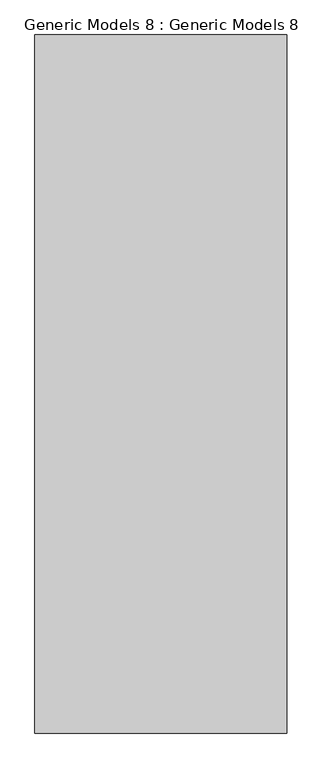
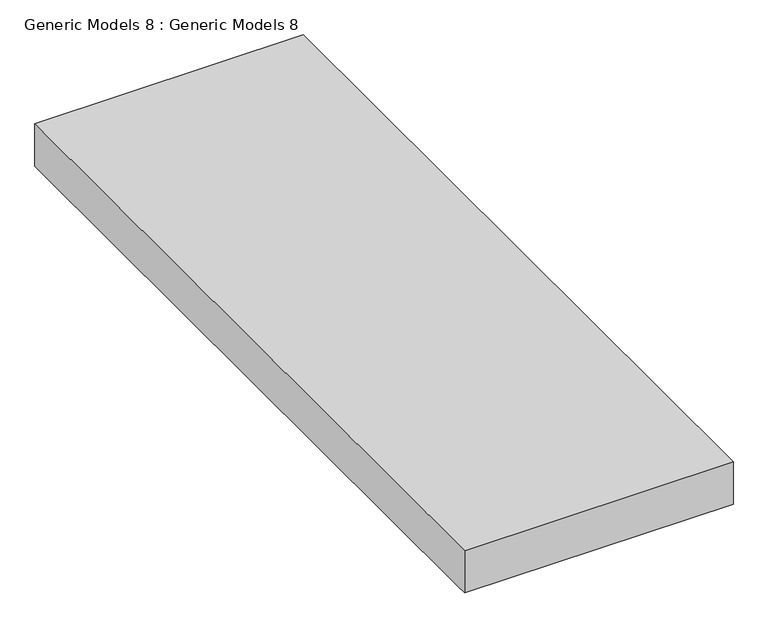
"""IFC4 building model written with IfcOpenShell, lengths in millimetres: proxy geometry, Generic Models 8 : Generic Models 8."""

from ifc_helpers import new_model, si_unit, frame, origin, place, context, project, spatial, polyline, outline, extrude, source, transform, mapped, element, save


def generic_models_8_generic_models_8_8680fe62(model_context):
    return source(origin(), model_context, "Body", "SweptSolid", [
        extrude(outline(polyline([(10620.4944012, 2190.75), (10595.0944012, 2190.75), (8956.7944012, 2190.75), (8931.3944012, 2190.75), (8931.3944012, 2292.35), (10620.4944012, 2292.35), (10620.4944012, 2190.75)])), frame((-506.5519453, 0.0, 0.0), z_axis=(1.0, 0.0, 0.0), x_axis=(0.0, 1.0, 0.0)), (0.0, 0.0, 1.0), 609.6),
    ])


if __name__ == "__main__":
    model = new_model("IFC4")
    model_context = context("Model", 3, world=origin())
    ifc_project = project(units=[si_unit("LENGTHUNIT", "METRE", prefix="MILLI")], contexts=[model_context])
    site = spatial("IfcSite", under=ifc_project)
    building = spatial("IfcBuilding", under=site)
    placement = place(None, origin())
    generic_models_8_generic_models_8_shape = generic_models_8_generic_models_8_8680fe62(model_context)
    element("IfcBuildingElementProxy", 1, Name="Generic Models 8 : Generic Models 8", ObjectType="Generic Models 8 : Generic Models 8", at=placement, inside=building, context=model_context, shape_type="MappedRepresentation", body=[
        mapped(generic_models_8_generic_models_8_shape, transform((0.0, 0.0, 0.0), x_axis=(1.0, 0.0, 0.0), y_axis=(0.0, 1.0, 0.0), z_axis=(0.0, 0.0, 1.0))),
    ])
    save(model, "model.ifc")
